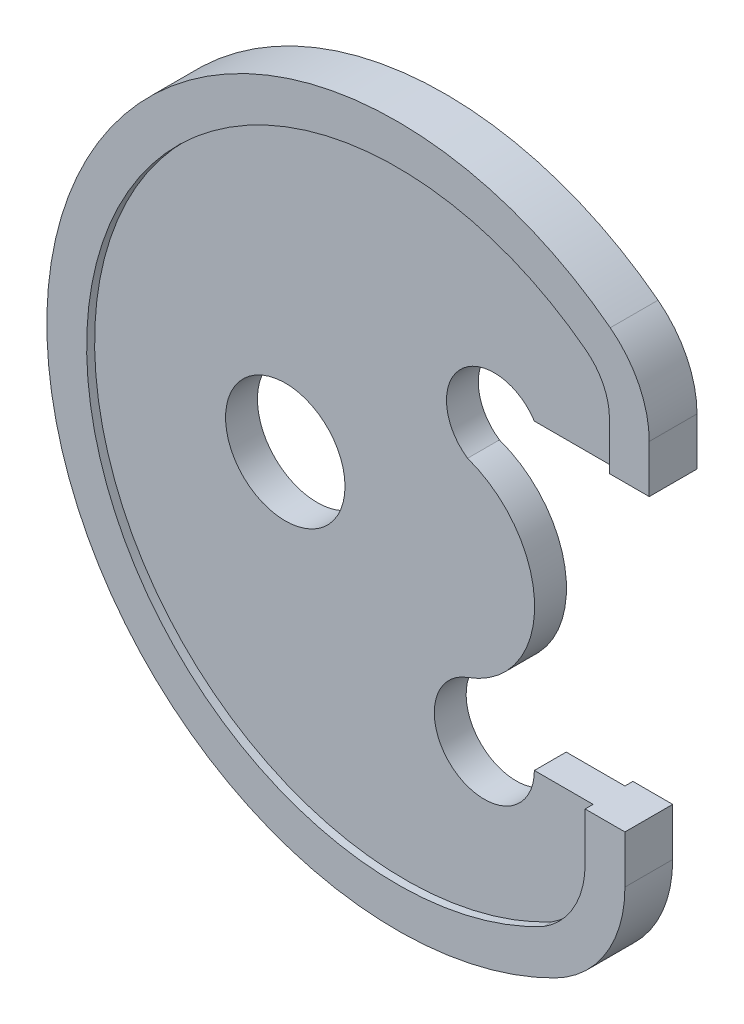
ISO-10303-21;
HEADER;
FILE_DESCRIPTION(('STEP AP214'),'2;1');
FILE_NAME('part.step','',(''),(''),'','','');
FILE_SCHEMA(('AUTOMOTIVE_DESIGN { 1 0 10303 214 1 1 1 1 }'));
ENDSEC;
DATA;
#1=APPLICATION_CONTEXT('core data for automotive mechanical design processes');
#2=APPLICATION_PROTOCOL_DEFINITION('international standard','automotive_design',2000,#1);
#3=PRODUCT_CONTEXT('',#1,'mechanical');
#4=PRODUCT('Part','Part','',(#3));
#5=PRODUCT_RELATED_PRODUCT_CATEGORY('part','',(#4));
#6=PRODUCT_DEFINITION_FORMATION('','',#4);
#7=PRODUCT_DEFINITION_CONTEXT('part definition',#1,'design');
#8=PRODUCT_DEFINITION('design','',#6,#7);
#9=PRODUCT_DEFINITION_SHAPE('','',#8);
#10=(LENGTH_UNIT() NAMED_UNIT(*) SI_UNIT(.MILLI.,.METRE.));
#11=(NAMED_UNIT(*) PLANE_ANGLE_UNIT() SI_UNIT($,.RADIAN.));
#12=(NAMED_UNIT(*) SI_UNIT($,.STERADIAN.) SOLID_ANGLE_UNIT());
#13=UNCERTAINTY_MEASURE_WITH_UNIT(LENGTH_MEASURE(1.E-05),#10,'distance_accuracy_value','');
#14=(GEOMETRIC_REPRESENTATION_CONTEXT(3) GLOBAL_UNCERTAINTY_ASSIGNED_CONTEXT((#13)) GLOBAL_UNIT_ASSIGNED_CONTEXT((#10,
#11,#12)) REPRESENTATION_CONTEXT('',''));
#15=CARTESIAN_POINT('',(0.,0.,0.));
#16=DIRECTION('',(0.,0.,1.));
#17=DIRECTION('',(1.,0.,0.));
#18=AXIS2_PLACEMENT_3D('',#15,#16,#17);
#19=CARTESIAN_POINT('',(7.23914147945783,-2.31584053817789,-4.));
#20=DIRECTION('',(0.,0.,1.));
#21=DIRECTION('',(1.,0.,0.));
#22=AXIS2_PLACEMENT_3D('',#19,#20,#21);
#23=CYLINDRICAL_SURFACE('',#22,25.2954749771281);
#24=CARTESIAN_POINT('',(7.23914147945783,-2.31584053817789,4.));
#25=DIRECTION('',(0.,0.,1.));
#26=DIRECTION('',(1.,0.,0.));
#27=AXIS2_PLACEMENT_3D('',#24,#25,#26);
#28=CIRCLE('',#27,25.2954749771281);
#29=CARTESIAN_POINT('',(15.6965465818434,21.523902607516,4.));
#30=VERTEX_POINT('',#29);
#31=CARTESIAN_POINT('',(15.6965465818434,-26.1555836838718,4.));
#32=VERTEX_POINT('',#31);
#33=EDGE_CURVE('E342',#30,#32,#28,.F.);
#34=ORIENTED_EDGE('',*,*,#33,.T.);
#35=DIRECTION('',(0.,0.,1.));
#36=VECTOR('',#35,1.);
#37=CARTESIAN_POINT('',(15.6965465818434,-26.1555836838718,-4.));
#38=LINE('',#37,#36);
#39=CARTESIAN_POINT('',(15.6965465818434,-26.1555836838718,-4.));
#40=VERTEX_POINT('',#39);
#41=EDGE_CURVE('E290',#40,#32,#38,.T.);
#42=ORIENTED_EDGE('',*,*,#41,.F.);
#43=CARTESIAN_POINT('',(7.23914147945783,-2.31584053817789,-4.));
#44=DIRECTION('',(0.,0.,1.));
#45=DIRECTION('',(1.,0.,0.));
#46=AXIS2_PLACEMENT_3D('',#43,#44,#45);
#47=CIRCLE('',#46,25.2954749771281);
#48=CARTESIAN_POINT('',(15.6965465818434,21.523902607516,-4.));
#49=VERTEX_POINT('',#48);
#50=EDGE_CURVE('E294',#40,#49,#47,.T.);
#51=ORIENTED_EDGE('',*,*,#50,.T.);
#52=DIRECTION('',(0.,0.,1.));
#53=VECTOR('',#52,1.);
#54=CARTESIAN_POINT('',(15.6965465818434,21.523902607516,-4.));
#55=LINE('',#54,#53);
#56=EDGE_CURVE('E288',#49,#30,#55,.T.);
#57=ORIENTED_EDGE('',*,*,#56,.T.);
#58=EDGE_LOOP('',(#34,#42,#51,#57));
#59=FACE_BOUND('',#58,.T.);
#60=ADVANCED_FACE('F37',(#59),#23,.T.);
#61=CARTESIAN_POINT('',(19.8984805697479,-38.,-4.));
#62=DIRECTION('',(0.,0.,1.));
#63=DIRECTION('',(1.,0.,0.));
#64=AXIS2_PLACEMENT_3D('',#61,#62,#63);
#65=CYLINDRICAL_SURFACE('',#64,12.5676746897933);
#66=ORIENTED_EDGE('',*,*,#41,.T.);
#67=CARTESIAN_POINT('',(19.8984805697479,-38.,4.));
#68=DIRECTION('',(0.,0.,1.));
#69=DIRECTION('',(1.,0.,0.));
#70=AXIS2_PLACEMENT_3D('',#67,#68,#69);
#71=CIRCLE('',#70,12.5676746897933);
#72=CARTESIAN_POINT('',(32.4661552595412,-38.,4.));
#73=VERTEX_POINT('',#72);
#74=EDGE_CURVE('E347',#73,#32,#71,.F.);
#75=ORIENTED_EDGE('',*,*,#74,.F.);
#76=DIRECTION('',(0.,0.,1.));
#77=VECTOR('',#76,1.);
#78=CARTESIAN_POINT('',(32.4661552595412,-38.,-4.));
#79=LINE('',#78,#77);
#80=CARTESIAN_POINT('',(32.4661552595412,-38.,-4.));
#81=VERTEX_POINT('',#80);
#82=EDGE_CURVE('E266',#81,#73,#79,.T.);
#83=ORIENTED_EDGE('',*,*,#82,.F.);
#84=CARTESIAN_POINT('',(19.8984805697479,-38.,-4.));
#85=DIRECTION('',(0.,0.,-1.));
#86=DIRECTION('',(-1.,0.,0.));
#87=AXIS2_PLACEMENT_3D('',#84,#85,#86);
#88=CIRCLE('',#87,12.5676746897933);
#89=EDGE_CURVE('E296',#81,#40,#88,.T.);
#90=ORIENTED_EDGE('',*,*,#89,.T.);
#91=EDGE_LOOP('',(#66,#75,#83,#90));
#92=FACE_BOUND('',#91,.T.);
#93=ADVANCED_FACE('F389',(#92),#65,.F.);
#94=CARTESIAN_POINT('',(53.3275357934736,38.,6.));
#95=DIRECTION('',(0.,1.,0.));
#96=DIRECTION('',(0.,0.,1.));
#97=AXIS2_PLACEMENT_3D('',#94,#95,#96);
#98=PLANE('',#97);
#99=DIRECTION('',(0.,0.,1.));
#100=VECTOR('',#99,1.);
#101=CARTESIAN_POINT('',(53.3275357934736,38.,4.));
#102=LINE('',#101,#100);
#103=CARTESIAN_POINT('',(53.3275357934736,38.,4.));
#104=VERTEX_POINT('',#103);
#105=CARTESIAN_POINT('',(53.3275357934736,38.,6.));
#106=VERTEX_POINT('',#105);
#107=EDGE_CURVE('E265',#104,#106,#102,.T.);
#108=ORIENTED_EDGE('',*,*,#107,.F.);
#109=DIRECTION('',(1.,0.,0.));
#110=VECTOR('',#109,1.);
#111=CARTESIAN_POINT('',(0.,38.,4.));
#112=LINE('',#111,#110);
#113=CARTESIAN_POINT('',(32.4661552595412,38.,4.));
#114=VERTEX_POINT('',#113);
#115=EDGE_CURVE('E313',#114,#104,#112,.T.);
#116=ORIENTED_EDGE('',*,*,#115,.F.);
#117=DIRECTION('',(0.,0.,1.));
#118=VECTOR('',#117,1.);
#119=CARTESIAN_POINT('',(32.4661552595412,38.,-4.));
#120=LINE('',#119,#118);
#121=CARTESIAN_POINT('',(32.4661552595412,38.,-4.));
#122=VERTEX_POINT('',#121);
#123=EDGE_CURVE('E158',#122,#114,#120,.T.);
#124=ORIENTED_EDGE('',*,*,#123,.F.);
#125=DIRECTION('',(1.,0.,0.));
#126=VECTOR('',#125,1.);
#127=CARTESIAN_POINT('',(53.3275357934736,38.,-4.));
#128=LINE('',#127,#126);
#129=CARTESIAN_POINT('',(53.3275357934736,38.,-4.));
#130=VERTEX_POINT('',#129);
#131=EDGE_CURVE('E260',#122,#130,#128,.T.);
#132=ORIENTED_EDGE('',*,*,#131,.T.);
#133=DIRECTION('',(0.,0.,-1.));
#134=VECTOR('',#133,1.);
#135=CARTESIAN_POINT('',(53.3275357934736,38.,6.));
#136=LINE('',#135,#134);
#137=CARTESIAN_POINT('',(53.3275357934736,38.,-6.));
#138=VERTEX_POINT('',#137);
#139=EDGE_CURVE('E188',#130,#138,#136,.T.);
#140=ORIENTED_EDGE('',*,*,#139,.T.);
#141=DIRECTION('',(1.,0.,0.));
#142=VECTOR('',#141,1.);
#143=CARTESIAN_POINT('',(53.3275357934736,38.,-6.));
#144=LINE('',#143,#142);
#145=CARTESIAN_POINT('',(63.3275357934736,38.,-6.));
#146=VERTEX_POINT('',#145);
#147=EDGE_CURVE('E179',#138,#146,#144,.T.);
#148=ORIENTED_EDGE('',*,*,#147,.T.);
#149=DIRECTION('',(0.,0.,-1.));
#150=VECTOR('',#149,1.);
#151=CARTESIAN_POINT('',(63.3275357934736,38.,6.));
#152=LINE('',#151,#150);
#153=CARTESIAN_POINT('',(63.3275357934736,38.,6.));
#154=VERTEX_POINT('',#153);
#155=EDGE_CURVE('E150',#154,#146,#152,.T.);
#156=ORIENTED_EDGE('',*,*,#155,.F.);
#157=DIRECTION('',(1.,0.,0.));
#158=VECTOR('',#157,1.);
#159=CARTESIAN_POINT('',(53.3275357934736,38.,6.));
#160=LINE('',#159,#158);
#161=EDGE_CURVE('E135',#106,#154,#160,.T.);
#162=ORIENTED_EDGE('',*,*,#161,.F.);
#163=EDGE_LOOP('',(#108,#116,#124,#132,#140,#148,#156,#162));
#164=FACE_BOUND('',#163,.T.);
#165=ADVANCED_FACE('F269',(#164),#98,.F.);
#166=CARTESIAN_POINT('',(25.2190404258369,-50.,6.));
#167=DIRECTION('',(0.,0.,1.));
#168=DIRECTION('',(1.,0.,0.));
#169=AXIS2_PLACEMENT_3D('',#166,#167,#168);
#170=PLANE('',#169);
#171=CARTESIAN_POINT('',(38.3275357934736,50.,6.));
#172=DIRECTION('',(0.,0.,1.));
#173=DIRECTION('',(1.,0.,0.));
#174=AXIS2_PLACEMENT_3D('',#171,#172,#173);
#175=CIRCLE('',#174,15.);
#176=CARTESIAN_POINT('',(53.3275357934736,50.,6.));
#177=VERTEX_POINT('',#176);
#178=CARTESIAN_POINT('',(47.4531395538245,61.9047619047619,6.));
#179=VERTEX_POINT('',#178);
#180=EDGE_CURVE('E337',#177,#179,#175,.T.);
#181=ORIENTED_EDGE('',*,*,#180,.F.);
#182=DIRECTION('',(0.,-1.,0.));
#183=VECTOR('',#182,1.);
#184=CARTESIAN_POINT('',(53.3275357934736,0.,6.));
#185=LINE('',#184,#183);
#186=EDGE_CURVE('E339',#177,#106,#185,.T.);
#187=ORIENTED_EDGE('',*,*,#186,.T.);
#188=ORIENTED_EDGE('',*,*,#161,.T.);
#189=DIRECTION('',(0.,1.,0.));
#190=VECTOR('',#189,1.);
#191=CARTESIAN_POINT('',(63.3275357934736,50.,6.));
#192=LINE('',#191,#190);
#193=CARTESIAN_POINT('',(63.3275357934736,50.,6.));
#194=VERTEX_POINT('',#193);
#195=EDGE_CURVE('E127',#154,#194,#192,.T.);
#196=ORIENTED_EDGE('',*,*,#195,.T.);
#197=CARTESIAN_POINT('',(38.3275357934736,50.,6.));
#198=DIRECTION('',(0.,0.,1.));
#199=DIRECTION('',(1.,0.,0.));
#200=AXIS2_PLACEMENT_3D('',#197,#198,#199);
#201=CIRCLE('',#200,25.);
#202=CARTESIAN_POINT('',(53.5368753940584,69.8412698412698,6.));
#203=VERTEX_POINT('',#202);
#204=EDGE_CURVE('E131',#194,#203,#201,.T.);
#205=ORIENTED_EDGE('',*,*,#204,.T.);
#206=CARTESIAN_POINT('',(0.,0.,6.));
#207=DIRECTION('',(0.,0.,1.));
#208=DIRECTION('',(1.,0.,0.));
#209=AXIS2_PLACEMENT_3D('',#206,#207,#208);
#210=CIRCLE('',#209,88.);
#211=CARTESIAN_POINT('',(39.6299206691723,-78.5714285714286,6.));
#212=VERTEX_POINT('',#211);
#213=EDGE_CURVE('E61',#203,#212,#210,.T.);
#214=ORIENTED_EDGE('',*,*,#213,.T.);
#215=CARTESIAN_POINT('',(25.2190404258369,-50.,6.));
#216=DIRECTION('',(0.,0.,1.));
#217=DIRECTION('',(1.,0.,0.));
#218=AXIS2_PLACEMENT_3D('',#215,#216,#217);
#219=CIRCLE('',#218,32.);
#220=CARTESIAN_POINT('',(57.219040425837,-50.,6.));
#221=VERTEX_POINT('',#220);
#222=EDGE_CURVE('E187',#212,#221,#219,.T.);
#223=ORIENTED_EDGE('',*,*,#222,.T.);
#224=DIRECTION('',(0.,1.,0.));
#225=VECTOR('',#224,1.);
#226=CARTESIAN_POINT('',(57.219040425837,-50.,6.));
#227=LINE('',#226,#225);
#228=CARTESIAN_POINT('',(57.219040425837,-38.,6.));
#229=VERTEX_POINT('',#228);
#230=EDGE_CURVE('E120',#221,#229,#227,.T.);
#231=ORIENTED_EDGE('',*,*,#230,.T.);
#232=DIRECTION('',(-1.,0.,0.));
#233=VECTOR('',#232,1.);
#234=CARTESIAN_POINT('',(47.2190404258369,-38.,6.));
#235=LINE('',#234,#233);
#236=CARTESIAN_POINT('',(47.2190404258369,-38.,6.));
#237=VERTEX_POINT('',#236);
#238=EDGE_CURVE('E208',#229,#237,#235,.T.);
#239=ORIENTED_EDGE('',*,*,#238,.T.);
#240=DIRECTION('',(0.,1.,0.));
#241=VECTOR('',#240,1.);
#242=CARTESIAN_POINT('',(47.2190404258369,0.,6.));
#243=LINE('',#242,#241);
#244=CARTESIAN_POINT('',(47.2190404258369,-50.,6.));
#245=VERTEX_POINT('',#244);
#246=EDGE_CURVE('E326',#245,#237,#243,.T.);
#247=ORIENTED_EDGE('',*,*,#246,.F.);
#248=CARTESIAN_POINT('',(25.0856082022296,-50.,6.));
#249=DIRECTION('',(0.,0.,1.));
#250=DIRECTION('',(1.,0.,0.));
#251=AXIS2_PLACEMENT_3D('',#248,#249,#250);
#252=CIRCLE('',#251,22.1334322236073);
#253=CARTESIAN_POINT('',(36.8667298988786,-68.7375023299736,6.));
#254=VERTEX_POINT('',#253);
#255=EDGE_CURVE('E330',#245,#254,#252,.F.);
#256=ORIENTED_EDGE('',*,*,#255,.T.);
#257=CARTESIAN_POINT('',(0.,0.,6.));
#258=DIRECTION('',(0.,0.,1.));
#259=DIRECTION('',(1.,0.,0.));
#260=AXIS2_PLACEMENT_3D('',#257,#258,#259);
#261=CIRCLE('',#260,78.);
#262=EDGE_CURVE('E334',#179,#254,#261,.T.);
#263=ORIENTED_EDGE('',*,*,#262,.F.);
#264=EDGE_LOOP('',(#181,#187,#188,#196,#205,#214,#223,#231,#239,#247,#256,#263));
#265=FACE_BOUND('',#264,.T.);
#266=ADVANCED_FACE('F126',(#265),#170,.T.);
#267=CARTESIAN_POINT('',(22.3892096842652,31.4842369692471,-4.));
#268=DIRECTION('',(0.,0.,1.));
#269=DIRECTION('',(1.,0.,0.));
#270=AXIS2_PLACEMENT_3D('',#267,#268,#269);
#271=CYLINDRICAL_SURFACE('',#270,12.);
#272=ORIENTED_EDGE('',*,*,#123,.T.);
#273=CARTESIAN_POINT('',(22.3892096842652,31.4842369692471,4.));
#274=DIRECTION('',(0.,0.,1.));
#275=DIRECTION('',(1.,0.,0.));
#276=AXIS2_PLACEMENT_3D('',#273,#274,#275);
#277=CIRCLE('',#276,12.);
#278=EDGE_CURVE('E341',#114,#30,#277,.T.);
#279=ORIENTED_EDGE('',*,*,#278,.T.);
#280=ORIENTED_EDGE('',*,*,#56,.F.);
#281=CARTESIAN_POINT('',(22.3892096842652,31.4842369692471,-4.));
#282=DIRECTION('',(0.,0.,-1.));
#283=DIRECTION('',(1.,0.,0.));
#284=AXIS2_PLACEMENT_3D('',#281,#282,#283);
#285=CIRCLE('',#284,12.);
#286=EDGE_CURVE('E268',#49,#122,#285,.T.);
#287=ORIENTED_EDGE('',*,*,#286,.T.);
#288=EDGE_LOOP('',(#272,#279,#280,#287));
#289=FACE_BOUND('',#288,.T.);
#290=ADVANCED_FACE('F388',(#289),#271,.F.);
#291=CARTESIAN_POINT('',(47.2190404258369,-50.,6.));
#292=DIRECTION('',(1.,0.,0.));
#293=DIRECTION('',(0.,1.,0.));
#294=AXIS2_PLACEMENT_3D('',#291,#292,#293);
#295=PLANE('',#294);
#296=DIRECTION('',(0.,1.,0.));
#297=VECTOR('',#296,1.);
#298=CARTESIAN_POINT('',(47.2190404258369,-38.,-4.));
#299=LINE('',#298,#297);
#300=CARTESIAN_POINT('',(47.2190404258369,-50.,-4.));
#301=VERTEX_POINT('',#300);
#302=CARTESIAN_POINT('',(47.2190404258369,-38.,-4.));
#303=VERTEX_POINT('',#302);
#304=EDGE_CURVE('E224',#301,#303,#299,.T.);
#305=ORIENTED_EDGE('',*,*,#304,.T.);
#306=DIRECTION('',(0.,0.,-1.));
#307=VECTOR('',#306,1.);
#308=CARTESIAN_POINT('',(47.2190404258369,-38.,6.));
#309=LINE('',#308,#307);
#310=CARTESIAN_POINT('',(47.2190404258369,-38.,-6.));
#311=VERTEX_POINT('',#310);
#312=EDGE_CURVE('E200',#303,#311,#309,.T.);
#313=ORIENTED_EDGE('',*,*,#312,.T.);
#314=DIRECTION('',(0.,-1.,0.));
#315=VECTOR('',#314,1.);
#316=CARTESIAN_POINT('',(47.2190404258369,-50.,-6.));
#317=LINE('',#316,#315);
#318=CARTESIAN_POINT('',(47.2190404258369,-50.,-6.));
#319=VERTEX_POINT('',#318);
#320=EDGE_CURVE('E164',#311,#319,#317,.T.);
#321=ORIENTED_EDGE('',*,*,#320,.T.);
#322=DIRECTION('',(0.,0.,-1.));
#323=VECTOR('',#322,1.);
#324=CARTESIAN_POINT('',(47.2190404258369,-50.,6.));
#325=LINE('',#324,#323);
#326=EDGE_CURVE('E199',#301,#319,#325,.T.);
#327=ORIENTED_EDGE('',*,*,#326,.F.);
#328=EDGE_LOOP('',(#305,#313,#321,#327));
#329=FACE_BOUND('',#328,.T.);
#330=ADVANCED_FACE('F218',(#329),#295,.F.);
#331=CARTESIAN_POINT('',(25.2190404258369,-50.,6.));
#332=DIRECTION('',(0.,0.,-1.));
#333=DIRECTION('',(-1.,0.,0.));
#334=AXIS2_PLACEMENT_3D('',#331,#332,#333);
#335=CYLINDRICAL_SURFACE('',#334,22.);
#336=CARTESIAN_POINT('',(25.2190404258369,-50.,-4.));
#337=DIRECTION('',(0.,0.,1.));
#338=DIRECTION('',(1.,0.,0.));
#339=AXIS2_PLACEMENT_3D('',#336,#337,#338);
#340=CIRCLE('',#339,22.);
#341=CARTESIAN_POINT('',(35.12652059313,-69.6428571428572,-4.));
#342=VERTEX_POINT('',#341);
#343=EDGE_CURVE('E303',#342,#301,#340,.T.);
#344=ORIENTED_EDGE('',*,*,#343,.T.);
#345=ORIENTED_EDGE('',*,*,#326,.T.);
#346=CARTESIAN_POINT('',(25.2190404258369,-50.,-6.));
#347=DIRECTION('',(0.,0.,-1.));
#348=DIRECTION('',(1.,0.,0.));
#349=AXIS2_PLACEMENT_3D('',#346,#347,#348);
#350=CIRCLE('',#349,22.);
#351=CARTESIAN_POINT('',(35.12652059313,-69.6428571428572,-6.));
#352=VERTEX_POINT('',#351);
#353=EDGE_CURVE('E166',#319,#352,#350,.T.);
#354=ORIENTED_EDGE('',*,*,#353,.T.);
#355=DIRECTION('',(0.,0.,-1.));
#356=VECTOR('',#355,1.);
#357=CARTESIAN_POINT('',(35.12652059313,-69.6428571428572,6.));
#358=LINE('',#357,#356);
#359=EDGE_CURVE('E196',#342,#352,#358,.T.);
#360=ORIENTED_EDGE('',*,*,#359,.F.);
#361=EDGE_LOOP('',(#344,#345,#354,#360));
#362=FACE_BOUND('',#361,.T.);
#363=ADVANCED_FACE('F419',(#362),#335,.F.);
#364=CARTESIAN_POINT('',(0.,0.,6.));
#365=DIRECTION('',(0.,0.,-1.));
#366=DIRECTION('',(-1.,0.,0.));
#367=AXIS2_PLACEMENT_3D('',#364,#365,#366);
#368=CYLINDRICAL_SURFACE('',#367,78.);
#369=CARTESIAN_POINT('',(0.,0.,-4.));
#370=DIRECTION('',(0.,0.,1.));
#371=DIRECTION('',(1.,0.,0.));
#372=AXIS2_PLACEMENT_3D('',#369,#370,#371);
#373=CIRCLE('',#372,78.);
#374=CARTESIAN_POINT('',(47.4531395538245,61.9047619047619,-4.));
#375=VERTEX_POINT('',#374);
#376=EDGE_CURVE('E306',#375,#342,#373,.T.);
#377=ORIENTED_EDGE('',*,*,#376,.T.);
#378=ORIENTED_EDGE('',*,*,#359,.T.);
#379=CARTESIAN_POINT('',(0.,0.,-6.));
#380=DIRECTION('',(0.,0.,-1.));
#381=DIRECTION('',(1.,0.,0.));
#382=AXIS2_PLACEMENT_3D('',#379,#380,#381);
#383=CIRCLE('',#382,78.);
#384=CARTESIAN_POINT('',(47.4531395538245,61.9047619047619,-6.));
#385=VERTEX_POINT('',#384);
#386=EDGE_CURVE('E171',#352,#385,#383,.T.);
#387=ORIENTED_EDGE('',*,*,#386,.T.);
#388=DIRECTION('',(0.,0.,-1.));
#389=VECTOR('',#388,1.);
#390=CARTESIAN_POINT('',(47.4531395538245,61.9047619047619,6.));
#391=LINE('',#390,#389);
#392=EDGE_CURVE('E191',#375,#385,#391,.T.);
#393=ORIENTED_EDGE('',*,*,#392,.F.);
#394=EDGE_LOOP('',(#377,#378,#387,#393));
#395=FACE_BOUND('',#394,.T.);
#396=ADVANCED_FACE('F420',(#395),#368,.F.);
#397=CARTESIAN_POINT('',(38.3275357934736,50.,6.));
#398=DIRECTION('',(0.,0.,-1.));
#399=DIRECTION('',(-1.,0.,0.));
#400=AXIS2_PLACEMENT_3D('',#397,#398,#399);
#401=CYLINDRICAL_SURFACE('',#400,15.);
#402=CARTESIAN_POINT('',(38.3275357934736,50.,-4.));
#403=DIRECTION('',(0.,0.,1.));
#404=DIRECTION('',(1.,0.,0.));
#405=AXIS2_PLACEMENT_3D('',#402,#403,#404);
#406=CIRCLE('',#405,15.);
#407=CARTESIAN_POINT('',(53.3275357934736,50.,-4.));
#408=VERTEX_POINT('',#407);
#409=EDGE_CURVE('E261',#408,#375,#406,.T.);
#410=ORIENTED_EDGE('',*,*,#409,.T.);
#411=ORIENTED_EDGE('',*,*,#392,.T.);
#412=CARTESIAN_POINT('',(38.3275357934736,50.,-6.));
#413=DIRECTION('',(0.,0.,-1.));
#414=DIRECTION('',(1.,0.,0.));
#415=AXIS2_PLACEMENT_3D('',#412,#413,#414);
#416=CIRCLE('',#415,15.);
#417=CARTESIAN_POINT('',(53.3275357934736,50.,-6.));
#418=VERTEX_POINT('',#417);
#419=EDGE_CURVE('E172',#385,#418,#416,.T.);
#420=ORIENTED_EDGE('',*,*,#419,.T.);
#421=DIRECTION('',(0.,0.,-1.));
#422=VECTOR('',#421,1.);
#423=CARTESIAN_POINT('',(53.3275357934736,50.,6.));
#424=LINE('',#423,#422);
#425=EDGE_CURVE('E195',#408,#418,#424,.T.);
#426=ORIENTED_EDGE('',*,*,#425,.F.);
#427=EDGE_LOOP('',(#410,#411,#420,#426));
#428=FACE_BOUND('',#427,.T.);
#429=ADVANCED_FACE('F418',(#428),#401,.F.);
#430=CARTESIAN_POINT('',(53.3275357934736,50.,6.));
#431=DIRECTION('',(1.,0.,0.));
#432=DIRECTION('',(0.,0.,-1.));
#433=AXIS2_PLACEMENT_3D('',#430,#431,#432);
#434=PLANE('',#433);
#435=DIRECTION('',(0.,1.,0.));
#436=VECTOR('',#435,1.);
#437=CARTESIAN_POINT('',(53.3275357934736,50.,-4.));
#438=LINE('',#437,#436);
#439=EDGE_CURVE('E251',#130,#408,#438,.T.);
#440=ORIENTED_EDGE('',*,*,#439,.T.);
#441=ORIENTED_EDGE('',*,*,#425,.T.);
#442=DIRECTION('',(0.,-1.,0.));
#443=VECTOR('',#442,1.);
#444=CARTESIAN_POINT('',(53.3275357934736,50.,-6.));
#445=LINE('',#444,#443);
#446=EDGE_CURVE('E180',#418,#138,#445,.T.);
#447=ORIENTED_EDGE('',*,*,#446,.T.);
#448=ORIENTED_EDGE('',*,*,#139,.F.);
#449=EDGE_LOOP('',(#440,#441,#447,#448));
#450=FACE_BOUND('',#449,.T.);
#451=ADVANCED_FACE('F275',(#450),#434,.F.);
#452=CARTESIAN_POINT('',(25.2190404258369,-50.,6.));
#453=DIRECTION('',(0.,0.,-1.));
#454=DIRECTION('',(-1.,0.,0.));
#455=AXIS2_PLACEMENT_3D('',#452,#453,#454);
#456=CYLINDRICAL_SURFACE('',#455,32.);
#457=CARTESIAN_POINT('',(25.2190404258369,-50.,-6.));
#458=DIRECTION('',(0.,0.,1.));
#459=DIRECTION('',(1.,0.,0.));
#460=AXIS2_PLACEMENT_3D('',#457,#458,#459);
#461=CIRCLE('',#460,32.);
#462=CARTESIAN_POINT('',(39.6299206691723,-78.5714285714286,-6.));
#463=VERTEX_POINT('',#462);
#464=CARTESIAN_POINT('',(57.219040425837,-50.,-6.));
#465=VERTEX_POINT('',#464);
#466=EDGE_CURVE('E157',#463,#465,#461,.T.);
#467=ORIENTED_EDGE('',*,*,#466,.T.);
#468=DIRECTION('',(0.,0.,-1.));
#469=VECTOR('',#468,1.);
#470=CARTESIAN_POINT('',(57.219040425837,-50.,6.));
#471=LINE('',#470,#469);
#472=EDGE_CURVE('E12',#221,#465,#471,.T.);
#473=ORIENTED_EDGE('',*,*,#472,.F.);
#474=ORIENTED_EDGE('',*,*,#222,.F.);
#475=DIRECTION('',(0.,0.,-1.));
#476=VECTOR('',#475,1.);
#477=CARTESIAN_POINT('',(39.6299206691723,-78.5714285714286,6.));
#478=LINE('',#477,#476);
#479=EDGE_CURVE('E152',#212,#463,#478,.T.);
#480=ORIENTED_EDGE('',*,*,#479,.T.);
#481=EDGE_LOOP('',(#467,#473,#474,#480));
#482=FACE_BOUND('',#481,.T.);
#483=ADVANCED_FACE('F45',(#482),#456,.T.);
#484=CARTESIAN_POINT('',(57.219040425837,-50.,6.));
#485=DIRECTION('',(-1.,0.,0.));
#486=DIRECTION('',(0.,0.,1.));
#487=AXIS2_PLACEMENT_3D('',#484,#485,#486);
#488=PLANE('',#487);
#489=DIRECTION('',(0.,1.,0.));
#490=VECTOR('',#489,1.);
#491=CARTESIAN_POINT('',(57.219040425837,-50.,-6.));
#492=LINE('',#491,#490);
#493=CARTESIAN_POINT('',(57.219040425837,-38.,-6.));
#494=VERTEX_POINT('',#493);
#495=EDGE_CURVE('E156',#465,#494,#492,.T.);
#496=ORIENTED_EDGE('',*,*,#495,.T.);
#497=DIRECTION('',(0.,0.,-1.));
#498=VECTOR('',#497,1.);
#499=CARTESIAN_POINT('',(57.219040425837,-38.,6.));
#500=LINE('',#499,#498);
#501=EDGE_CURVE('E48',#229,#494,#500,.T.);
#502=ORIENTED_EDGE('',*,*,#501,.F.);
#503=ORIENTED_EDGE('',*,*,#230,.F.);
#504=ORIENTED_EDGE('',*,*,#472,.T.);
#505=EDGE_LOOP('',(#496,#502,#503,#504));
#506=FACE_BOUND('',#505,.T.);
#507=ADVANCED_FACE('F508',(#506),#488,.F.);
#508=CARTESIAN_POINT('',(47.2190404258369,-38.,6.));
#509=DIRECTION('',(0.,-1.,0.));
#510=DIRECTION('',(0.,0.,-1.));
#511=AXIS2_PLACEMENT_3D('',#508,#509,#510);
#512=PLANE('',#511);
#513=DIRECTION('',(-1.,0.,0.));
#514=VECTOR('',#513,1.);
#515=CARTESIAN_POINT('',(0.,-38.,4.));
#516=LINE('',#515,#514);
#517=CARTESIAN_POINT('',(47.2190404258369,-38.,4.));
#518=VERTEX_POINT('',#517);
#519=EDGE_CURVE('E54',#518,#73,#516,.T.);
#520=ORIENTED_EDGE('',*,*,#519,.F.);
#521=DIRECTION('',(0.,0.,1.));
#522=VECTOR('',#521,1.);
#523=CARTESIAN_POINT('',(47.2190404258369,-38.,4.));
#524=LINE('',#523,#522);
#525=EDGE_CURVE('E324',#518,#237,#524,.T.);
#526=ORIENTED_EDGE('',*,*,#525,.T.);
#527=ORIENTED_EDGE('',*,*,#238,.F.);
#528=ORIENTED_EDGE('',*,*,#501,.T.);
#529=DIRECTION('',(-1.,0.,0.));
#530=VECTOR('',#529,1.);
#531=CARTESIAN_POINT('',(47.2190404258369,-38.,-6.));
#532=LINE('',#531,#530);
#533=EDGE_CURVE('E162',#494,#311,#532,.T.);
#534=ORIENTED_EDGE('',*,*,#533,.T.);
#535=ORIENTED_EDGE('',*,*,#312,.F.);
#536=DIRECTION('',(-1.,0.,0.));
#537=VECTOR('',#536,1.);
#538=CARTESIAN_POINT('',(47.2190404258369,-38.,-4.));
#539=LINE('',#538,#537);
#540=EDGE_CURVE('E226',#303,#81,#539,.T.);
#541=ORIENTED_EDGE('',*,*,#540,.T.);
#542=ORIENTED_EDGE('',*,*,#82,.T.);
#543=EDGE_LOOP('',(#520,#526,#527,#528,#534,#535,#541,#542));
#544=FACE_BOUND('',#543,.T.);
#545=ADVANCED_FACE('F203',(#544),#512,.F.);
#546=CARTESIAN_POINT('',(63.3275357934736,50.,6.));
#547=DIRECTION('',(-1.,0.,0.));
#548=DIRECTION('',(0.,0.,1.));
#549=AXIS2_PLACEMENT_3D('',#546,#547,#548);
#550=PLANE('',#549);
#551=DIRECTION('',(0.,1.,0.));
#552=VECTOR('',#551,1.);
#553=CARTESIAN_POINT('',(63.3275357934736,50.,-6.));
#554=LINE('',#553,#552);
#555=CARTESIAN_POINT('',(63.3275357934736,50.,-6.));
#556=VERTEX_POINT('',#555);
#557=EDGE_CURVE('E144',#146,#556,#554,.T.);
#558=ORIENTED_EDGE('',*,*,#557,.T.);
#559=DIRECTION('',(0.,0.,-1.));
#560=VECTOR('',#559,1.);
#561=CARTESIAN_POINT('',(63.3275357934736,50.,6.));
#562=LINE('',#561,#560);
#563=EDGE_CURVE('E142',#194,#556,#562,.T.);
#564=ORIENTED_EDGE('',*,*,#563,.F.);
#565=ORIENTED_EDGE('',*,*,#195,.F.);
#566=ORIENTED_EDGE('',*,*,#155,.T.);
#567=EDGE_LOOP('',(#558,#564,#565,#566));
#568=FACE_BOUND('',#567,.T.);
#569=ADVANCED_FACE('F145',(#568),#550,.F.);
#570=CARTESIAN_POINT('',(38.3275357934736,50.,6.));
#571=DIRECTION('',(0.,0.,-1.));
#572=DIRECTION('',(-1.,0.,0.));
#573=AXIS2_PLACEMENT_3D('',#570,#571,#572);
#574=CYLINDRICAL_SURFACE('',#573,25.);
#575=CARTESIAN_POINT('',(38.3275357934736,50.,-6.));
#576=DIRECTION('',(0.,0.,1.));
#577=DIRECTION('',(1.,0.,0.));
#578=AXIS2_PLACEMENT_3D('',#575,#576,#577);
#579=CIRCLE('',#578,25.);
#580=CARTESIAN_POINT('',(53.5368753940584,69.8412698412698,-6.));
#581=VERTEX_POINT('',#580);
#582=EDGE_CURVE('E182',#556,#581,#579,.T.);
#583=ORIENTED_EDGE('',*,*,#582,.T.);
#584=DIRECTION('',(0.,0.,-1.));
#585=VECTOR('',#584,1.);
#586=CARTESIAN_POINT('',(53.5368753940584,69.8412698412698,6.));
#587=LINE('',#586,#585);
#588=EDGE_CURVE('E149',#203,#581,#587,.T.);
#589=ORIENTED_EDGE('',*,*,#588,.F.);
#590=ORIENTED_EDGE('',*,*,#204,.F.);
#591=ORIENTED_EDGE('',*,*,#563,.T.);
#592=EDGE_LOOP('',(#583,#589,#590,#591));
#593=FACE_BOUND('',#592,.T.);
#594=ADVANCED_FACE('F148',(#593),#574,.T.);
#595=CARTESIAN_POINT('',(0.,0.,6.));
#596=DIRECTION('',(0.,0.,-1.));
#597=DIRECTION('',(-1.,0.,0.));
#598=AXIS2_PLACEMENT_3D('',#595,#596,#597);
#599=CYLINDRICAL_SURFACE('',#598,88.);
#600=CARTESIAN_POINT('',(0.,0.,-6.));
#601=DIRECTION('',(0.,0.,1.));
#602=DIRECTION('',(1.,0.,0.));
#603=AXIS2_PLACEMENT_3D('',#600,#601,#602);
#604=CIRCLE('',#603,88.);
#605=EDGE_CURVE('E107',#581,#463,#604,.T.);
#606=ORIENTED_EDGE('',*,*,#605,.T.);
#607=ORIENTED_EDGE('',*,*,#479,.F.);
#608=ORIENTED_EDGE('',*,*,#213,.F.);
#609=ORIENTED_EDGE('',*,*,#588,.T.);
#610=EDGE_LOOP('',(#606,#607,#608,#609));
#611=FACE_BOUND('',#610,.T.);
#612=ADVANCED_FACE('F442',(#611),#599,.T.);
#613=CARTESIAN_POINT('',(25.2190404258369,-50.,-6.));
#614=DIRECTION('',(0.,0.,1.));
#615=DIRECTION('',(1.,0.,0.));
#616=AXIS2_PLACEMENT_3D('',#613,#614,#615);
#617=PLANE('',#616);
#618=ORIENTED_EDGE('',*,*,#466,.F.);
#619=ORIENTED_EDGE('',*,*,#605,.F.);
#620=ORIENTED_EDGE('',*,*,#582,.F.);
#621=ORIENTED_EDGE('',*,*,#557,.F.);
#622=ORIENTED_EDGE('',*,*,#147,.F.);
#623=ORIENTED_EDGE('',*,*,#446,.F.);
#624=ORIENTED_EDGE('',*,*,#419,.F.);
#625=ORIENTED_EDGE('',*,*,#386,.F.);
#626=ORIENTED_EDGE('',*,*,#353,.F.);
#627=ORIENTED_EDGE('',*,*,#320,.F.);
#628=ORIENTED_EDGE('',*,*,#533,.F.);
#629=ORIENTED_EDGE('',*,*,#495,.F.);
#630=EDGE_LOOP('',(#618,#619,#620,#621,#622,#623,#624,#625,#626,#627,#628,#629));
#631=FACE_BOUND('',#630,.T.);
#632=ADVANCED_FACE('F214',(#631),#617,.F.);
#633=CARTESIAN_POINT('',(22.3892096842652,31.4842369692471,-4.));
#634=DIRECTION('',(0.,0.,1.));
#635=DIRECTION('',(1.,0.,0.));
#636=AXIS2_PLACEMENT_3D('',#633,#634,#635);
#637=PLANE('',#636);
#638=CARTESIAN_POINT('',(-30.1015194302521,0.,-4.));
#639=DIRECTION('',(0.,0.,1.));
#640=DIRECTION('',(1.,0.,0.));
#641=AXIS2_PLACEMENT_3D('',#638,#639,#640);
#642=CIRCLE('',#641,15.);
#643=CARTESIAN_POINT('',(-15.1015194302521,0.,-4.));
#644=VERTEX_POINT('',#643);
#645=EDGE_CURVE('E362',#644,#644,#642,.T.);
#646=ORIENTED_EDGE('',*,*,#645,.T.);
#647=EDGE_LOOP('',(#646));
#648=FACE_BOUND('',#647,.T.);
#649=ORIENTED_EDGE('',*,*,#439,.F.);
#650=ORIENTED_EDGE('',*,*,#131,.F.);
#651=ORIENTED_EDGE('',*,*,#286,.F.);
#652=ORIENTED_EDGE('',*,*,#50,.F.);
#653=ORIENTED_EDGE('',*,*,#89,.F.);
#654=ORIENTED_EDGE('',*,*,#540,.F.);
#655=ORIENTED_EDGE('',*,*,#304,.F.);
#656=ORIENTED_EDGE('',*,*,#343,.F.);
#657=ORIENTED_EDGE('',*,*,#376,.F.);
#658=ORIENTED_EDGE('',*,*,#409,.F.);
#659=EDGE_LOOP('',(#649,#650,#651,#652,#653,#654,#655,#656,#657,#658));
#660=FACE_BOUND('',#659,.T.);
#661=ADVANCED_FACE('F253',(#648,#660),#637,.F.);
#662=CARTESIAN_POINT('',(53.3275357934736,0.,4.));
#663=DIRECTION('',(-1.,0.,0.));
#664=DIRECTION('',(0.,0.,1.));
#665=AXIS2_PLACEMENT_3D('',#662,#663,#664);
#666=PLANE('',#665);
#667=ORIENTED_EDGE('',*,*,#186,.F.);
#668=DIRECTION('',(0.,0.,1.));
#669=VECTOR('',#668,1.);
#670=CARTESIAN_POINT('',(53.3275357934736,50.,4.));
#671=LINE('',#670,#669);
#672=CARTESIAN_POINT('',(53.3275357934736,50.,4.));
#673=VERTEX_POINT('',#672);
#674=EDGE_CURVE('E309',#673,#177,#671,.T.);
#675=ORIENTED_EDGE('',*,*,#674,.F.);
#676=DIRECTION('',(0.,-1.,0.));
#677=VECTOR('',#676,1.);
#678=CARTESIAN_POINT('',(53.3275357934736,0.,4.));
#679=LINE('',#678,#677);
#680=EDGE_CURVE('E328',#673,#104,#679,.T.);
#681=ORIENTED_EDGE('',*,*,#680,.T.);
#682=ORIENTED_EDGE('',*,*,#107,.T.);
#683=EDGE_LOOP('',(#667,#675,#681,#682));
#684=FACE_BOUND('',#683,.T.);
#685=ADVANCED_FACE('F461',(#684),#666,.T.);
#686=CARTESIAN_POINT('',(47.2190404258369,0.,4.));
#687=DIRECTION('',(1.,0.,0.));
#688=DIRECTION('',(0.,0.,-1.));
#689=AXIS2_PLACEMENT_3D('',#686,#687,#688);
#690=PLANE('',#689);
#691=ORIENTED_EDGE('',*,*,#246,.T.);
#692=ORIENTED_EDGE('',*,*,#525,.F.);
#693=DIRECTION('',(0.,1.,0.));
#694=VECTOR('',#693,1.);
#695=CARTESIAN_POINT('',(47.2190404258369,0.,4.));
#696=LINE('',#695,#694);
#697=CARTESIAN_POINT('',(47.2190404258369,-50.,4.));
#698=VERTEX_POINT('',#697);
#699=EDGE_CURVE('E350',#698,#518,#696,.T.);
#700=ORIENTED_EDGE('',*,*,#699,.F.);
#701=DIRECTION('',(0.,0.,1.));
#702=VECTOR('',#701,1.);
#703=CARTESIAN_POINT('',(47.2190404258369,-50.,4.));
#704=LINE('',#703,#702);
#705=EDGE_CURVE('E318',#698,#245,#704,.T.);
#706=ORIENTED_EDGE('',*,*,#705,.T.);
#707=EDGE_LOOP('',(#691,#692,#700,#706));
#708=FACE_BOUND('',#707,.T.);
#709=ADVANCED_FACE('F466',(#708),#690,.F.);
#710=CARTESIAN_POINT('',(25.0856082022296,-50.,4.));
#711=DIRECTION('',(0.,0.,1.));
#712=DIRECTION('',(1.,0.,0.));
#713=AXIS2_PLACEMENT_3D('',#710,#711,#712);
#714=CYLINDRICAL_SURFACE('',#713,22.1334322236073);
#715=ORIENTED_EDGE('',*,*,#255,.F.);
#716=ORIENTED_EDGE('',*,*,#705,.F.);
#717=CARTESIAN_POINT('',(25.0856082022296,-50.,4.));
#718=DIRECTION('',(0.,0.,1.));
#719=DIRECTION('',(1.,0.,0.));
#720=AXIS2_PLACEMENT_3D('',#717,#718,#719);
#721=CIRCLE('',#720,22.1334322236073);
#722=CARTESIAN_POINT('',(36.8667298988786,-68.7375023299736,4.));
#723=VERTEX_POINT('',#722);
#724=EDGE_CURVE('E355',#698,#723,#721,.F.);
#725=ORIENTED_EDGE('',*,*,#724,.T.);
#726=DIRECTION('',(0.,0.,1.));
#727=VECTOR('',#726,1.);
#728=CARTESIAN_POINT('',(36.8667298988786,-68.7375023299736,4.));
#729=LINE('',#728,#727);
#730=EDGE_CURVE('E320',#723,#254,#729,.T.);
#731=ORIENTED_EDGE('',*,*,#730,.T.);
#732=EDGE_LOOP('',(#715,#716,#725,#731));
#733=FACE_BOUND('',#732,.T.);
#734=ADVANCED_FACE('F476',(#733),#714,.F.);
#735=CARTESIAN_POINT('',(0.,0.,4.));
#736=DIRECTION('',(0.,0.,1.));
#737=DIRECTION('',(1.,0.,0.));
#738=AXIS2_PLACEMENT_3D('',#735,#736,#737);
#739=CYLINDRICAL_SURFACE('',#738,78.);
#740=ORIENTED_EDGE('',*,*,#262,.T.);
#741=ORIENTED_EDGE('',*,*,#730,.F.);
#742=CARTESIAN_POINT('',(0.,0.,4.));
#743=DIRECTION('',(0.,0.,1.));
#744=DIRECTION('',(1.,0.,0.));
#745=AXIS2_PLACEMENT_3D('',#742,#743,#744);
#746=CIRCLE('',#745,78.);
#747=CARTESIAN_POINT('',(47.4531395538245,61.9047619047619,4.));
#748=VERTEX_POINT('',#747);
#749=EDGE_CURVE('E353',#748,#723,#746,.T.);
#750=ORIENTED_EDGE('',*,*,#749,.F.);
#751=DIRECTION('',(0.,0.,1.));
#752=VECTOR('',#751,1.);
#753=CARTESIAN_POINT('',(47.4531395538245,61.9047619047619,4.));
#754=LINE('',#753,#752);
#755=EDGE_CURVE('E312',#748,#179,#754,.T.);
#756=ORIENTED_EDGE('',*,*,#755,.T.);
#757=EDGE_LOOP('',(#740,#741,#750,#756));
#758=FACE_BOUND('',#757,.T.);
#759=ADVANCED_FACE('F483',(#758),#739,.F.);
#760=CARTESIAN_POINT('',(38.3275357934736,50.,4.));
#761=DIRECTION('',(0.,0.,1.));
#762=DIRECTION('',(1.,0.,0.));
#763=AXIS2_PLACEMENT_3D('',#760,#761,#762);
#764=CYLINDRICAL_SURFACE('',#763,15.);
#765=ORIENTED_EDGE('',*,*,#180,.T.);
#766=ORIENTED_EDGE('',*,*,#755,.F.);
#767=CARTESIAN_POINT('',(38.3275357934736,50.,4.));
#768=DIRECTION('',(0.,0.,1.));
#769=DIRECTION('',(1.,0.,0.));
#770=AXIS2_PLACEMENT_3D('',#767,#768,#769);
#771=CIRCLE('',#770,15.);
#772=EDGE_CURVE('E356',#673,#748,#771,.T.);
#773=ORIENTED_EDGE('',*,*,#772,.F.);
#774=ORIENTED_EDGE('',*,*,#674,.T.);
#775=EDGE_LOOP('',(#765,#766,#773,#774));
#776=FACE_BOUND('',#775,.T.);
#777=ADVANCED_FACE('F380',(#776),#764,.F.);
#778=CARTESIAN_POINT('',(0.,0.,4.));
#779=DIRECTION('',(0.,0.,1.));
#780=DIRECTION('',(1.,0.,0.));
#781=AXIS2_PLACEMENT_3D('',#778,#779,#780);
#782=PLANE('',#781);
#783=CARTESIAN_POINT('',(-30.1015194302521,0.,4.));
#784=DIRECTION('',(0.,0.,1.));
#785=DIRECTION('',(1.,0.,0.));
#786=AXIS2_PLACEMENT_3D('',#783,#784,#785);
#787=CIRCLE('',#786,15.);
#788=CARTESIAN_POINT('',(-15.1015194302521,0.,4.));
#789=VERTEX_POINT('',#788);
#790=EDGE_CURVE('E368',#789,#789,#787,.T.);
#791=ORIENTED_EDGE('',*,*,#790,.F.);
#792=EDGE_LOOP('',(#791));
#793=FACE_BOUND('',#792,.T.);
#794=ORIENTED_EDGE('',*,*,#74,.T.);
#795=ORIENTED_EDGE('',*,*,#33,.F.);
#796=ORIENTED_EDGE('',*,*,#278,.F.);
#797=ORIENTED_EDGE('',*,*,#115,.T.);
#798=ORIENTED_EDGE('',*,*,#680,.F.);
#799=ORIENTED_EDGE('',*,*,#772,.T.);
#800=ORIENTED_EDGE('',*,*,#749,.T.);
#801=ORIENTED_EDGE('',*,*,#724,.F.);
#802=ORIENTED_EDGE('',*,*,#699,.T.);
#803=ORIENTED_EDGE('',*,*,#519,.T.);
#804=EDGE_LOOP('',(#794,#795,#796,#797,#798,#799,#800,#801,#802,#803));
#805=FACE_BOUND('',#804,.T.);
#806=ADVANCED_FACE('F374',(#793,#805),#782,.T.);
#807=CARTESIAN_POINT('',(-30.1015194302521,0.,-6.));
#808=DIRECTION('',(0.,0.,1.));
#809=DIRECTION('',(1.,0.,0.));
#810=AXIS2_PLACEMENT_3D('',#807,#808,#809);
#811=CYLINDRICAL_SURFACE('',#810,15.);
#812=ORIENTED_EDGE('',*,*,#790,.T.);
#813=EDGE_LOOP('',(#812));
#814=FACE_BOUND('',#813,.T.);
#815=ORIENTED_EDGE('',*,*,#645,.F.);
#816=EDGE_LOOP('',(#815));
#817=FACE_BOUND('',#816,.T.);
#818=ADVANCED_FACE('F375',(#814,#817),#811,.F.);
#819=CLOSED_SHELL('',(#60,#93,#165,#266,#290,#330,#363,#396,#429,#451,#483,#507,#545,#569,#594,
#612,#632,#661,#685,#709,#734,#759,#777,#806,#818));
#820=MANIFOLD_SOLID_BREP('B2',#819);
#821=ADVANCED_BREP_SHAPE_REPRESENTATION('',(#18,#820),#14);
#822=SHAPE_DEFINITION_REPRESENTATION(#9,#821);
ENDSEC;
END-ISO-10303-21;
